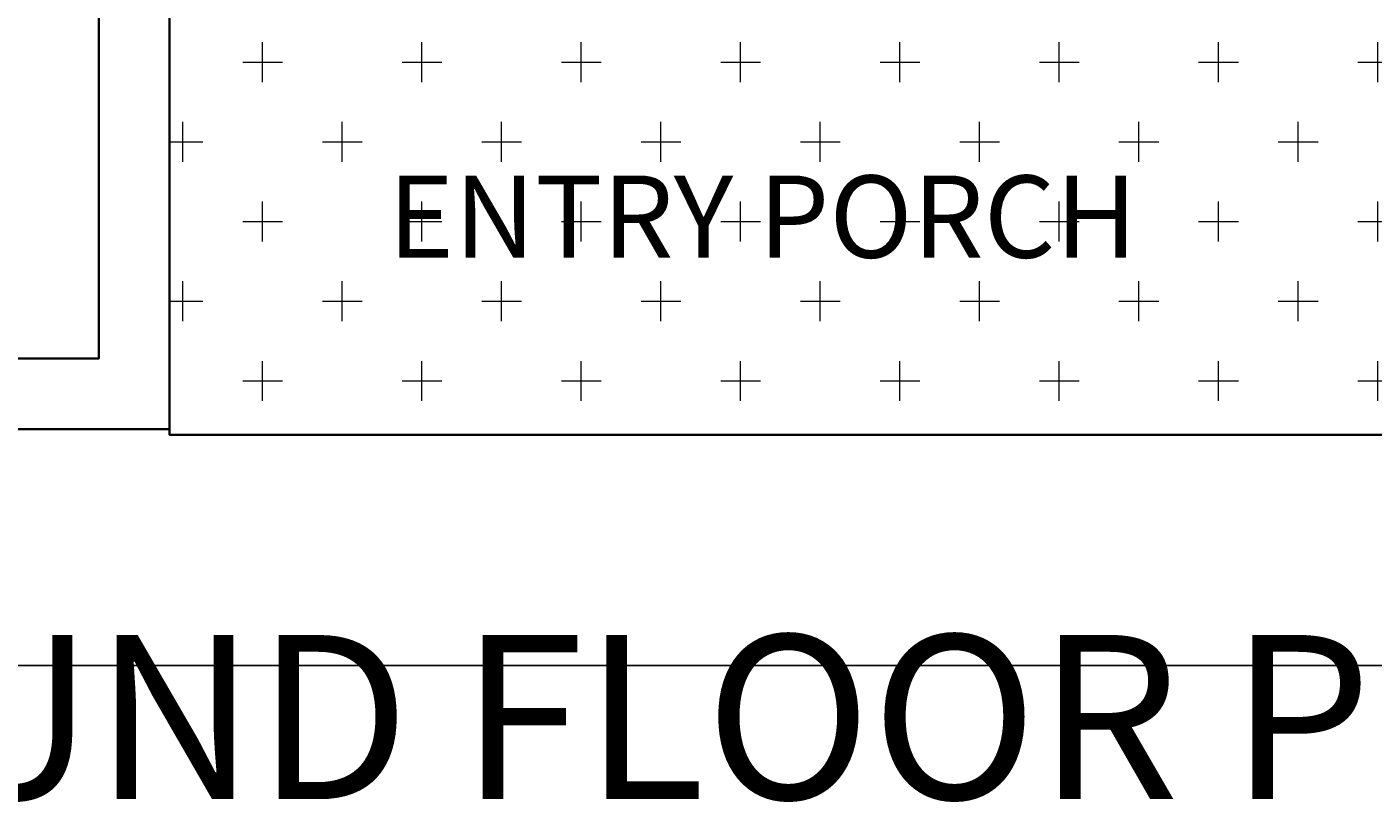
# Model space of a CAD drawing. Units: millimetres. Extents: x 19292 to 100733, y 12374 to 26974.
# Tile 2 of 24: x 26744 to 31036, y 12374 to 14845. Entities that reach past the tile are written whole.
import ezdxf

# ---------------------------------------------------------------- set-up
doc = ezdxf.new("R2010")
doc.units = ezdxf.units.MM
for name, color, linetype, lineweight in [('A-ANNO-DIMS', 2, 'Continuous', 18), ('A-ANNO-TEXT', 7, 'Continuous', 35), ('A-AREA-IDEN', 3, 'Continuous', 25), ('A-FLOR-PATT', 252, 'Continuous', 13), ('A-WALL', 7, 'Continuous', 35)]:
    doc.layers.add(name, color=color, linetype=linetype, lineweight=lineweight)
doc.styles.get("Standard").update_dxf_attribs({"font": 'arial.ttf'})
doc.dimstyles.get("Standard").update_dxf_attribs({"dimtxt": 0.18, "dimasz": 0.18, "dimexe": 0.18, "dimexo": 0.0625, "dimgap": 0.09, "dimtad": 0, "dimtih": 1, "dimtoh": 1, "dimdec": 4, "dimzin": 0, "dimdsep": 46, "dimtxsty": 'Standard', "dimcen": 0.09, "dimadec": 0, "dimazin": 0, "dimtfac": 1, "dimtdec": 4, "dimtofl": 0, "dimtmove": 0, "dimatfit": 3, "dimfxl": 1, "dimtolj": 1, "dimtzin": 0, "dimarcsym": 0})

# ---------------------------------------------------------------- blocks, each defined once
blk = doc.blocks.new('*D71')
at = {"layer": 'A-ANNO-DIMS', "color": 0, "lineweight": -2, "transparency": 16777216}
for p, q in [((26973.8, 17387.7), (26278.6, 17387.7)), ((26278.8, 17387.6), (26278.8, 15587.9)), ((26278.8, 13787.9), (26278.8, 15587.6)), ((26973.8, 13787.7), (26278.6, 13787.7))]:
    blk.add_line(p, q, dxfattribs=at)
at = {"layer": 'A-ANNO-DIMS', "color": 0, "transparency": 16777216}
for points in [[(26278.8, 17387.6), (26278.8, 17387.6), (26278.8, 17387.7)], [(26278.8, 13787.9), (26278.8, 13787.9), (26278.8, 13787.7)]]:
    blk.add_solid(points, dxfattribs=at)
at = {"layer": 'Defpoints', "color": 0, "transparency": 16777216}
for p in [(26278.8, 17387.7), (26973.8, 17387.7), (26973.8, 13787.7)]:
    blk.add_point(p, dxfattribs=at)
at = {"layer": 'A-ANNO-DIMS', "color": 0, "transparency": 16777216, "insert": (26278.8, 15587.7), "char_height": 0.18, "attachment_point": 5}
blk.add_mtext('\\A1;3600', dxfattribs=at)
blk = doc.blocks.new('*D79')
at = {"layer": 'A-ANNO-DIMS', "color": 0, "lineweight": -2, "transparency": 16777216}
for p, q in [((22694.1, 22860.7), (22694.1, 12808.8)), ((36144.2, 15985.7), (36144.2, 12808.8)), ((22694.3, 12809), (29418.7, 12809)), ((36144, 12809), (29419.6, 12809))]:
    blk.add_line(p, q, dxfattribs=at)
at = {"layer": 'A-ANNO-DIMS', "color": 0, "transparency": 16777216}
for points in [[(22694.3, 12809), (22694.3, 12809), (22694.1, 12809)], [(36144, 12809), (36144, 12809), (36144.2, 12809)]]:
    blk.add_solid(points, dxfattribs=at)
at = {"layer": 'Defpoints', "color": 0, "transparency": 16777216}
for p in [(22694.1, 22860.7), (36144.2, 15985.7), (36144.2, 12809)]:
    blk.add_point(p, dxfattribs=at)
at = {"layer": 'A-ANNO-DIMS', "color": 0, "transparency": 16777216, "insert": (29419.2, 12809), "char_height": 0.18, "attachment_point": 5}
blk.add_mtext('\\A1;13450', dxfattribs=at)
blk = doc.blocks.new('*D82')
at = {"layer": 'A-ANNO-DIMS', "color": 0, "lineweight": -2, "transparency": 16777216}
for p, q in [((27198.8, 13562.8), (27198.8, 23555.9)), ((27199, 23555.7), (29296.4, 23555.7)), ((31394.6, 23555.7), (29297.2, 23555.7)), ((31394.8, 13544.1), (31394.8, 23555.9))]:
    blk.add_line(p, q, dxfattribs=at)
at = {"layer": 'A-ANNO-DIMS', "color": 0, "transparency": 16777216}
for points in [[(27199, 23555.8), (27199, 23555.7), (27198.8, 23555.7)], [(31394.6, 23555.8), (31394.6, 23555.7), (31394.8, 23555.7)]]:
    blk.add_solid(points, dxfattribs=at)
at = {"layer": 'Defpoints', "color": 0, "transparency": 16777216}
for p in [(31394.8, 23555.7), (27198.8, 13562.7), (31394.8, 13544)]:
    blk.add_point(p, dxfattribs=at)
at = {"layer": 'A-ANNO-DIMS', "color": 0, "transparency": 16777216, "insert": (29296.8, 23555.7), "char_height": 0.18, "attachment_point": 5}
blk.add_mtext('\\A1;4196', dxfattribs=at)

msp = doc.modelspace()

# ---------------------------------------------------------------- hatches: boundary and pattern name
at = {"layer": 'A-FLOR-PATT'}
h = msp.add_hatch(dxfattribs=at)
h.set_pattern_fill('CROSS', color=256, scale=40)
h.paths.add_polyline_path([(31394.799, 14906.403), (31051.542, 14906.403), (29468.571, 14906.403), (27198.815, 14906.403), (27198.815, 13543.993), (31394.799, 13543.993)])
h.paths.add_polyline_path([(27828.096, 14036.581), (30629.164, 14036.581), (30629.164, 14443.478), (27828.096, 14443.478)], flags=24)

# ---------------------------------------------------------------- linework, layer by layer
at = {"layer": 'A-WALL'}
for points in [[(29548.571, 14906.403), (27198.815, 14906.403), (27198.815, 13562.748), (23348.815, 13562.748), (23348.815, 19010.725), (22694.132, 19010.725), (22694.132, 22860.725), (28369.132, 22860.725), (28369.132, 21460.725), (31169.132, 21460.725), (31169.132, 22460.725), (34419.132, 22460.725), (34419.132, 22208.026)], [(25756.145, 17387.748), (23573.815, 17387.748), (23573.815, 13787.748), (26973.815, 13787.748), (26973.815, 17387.748), (26656.145, 17387.748)], [(31051.542, 14906.403), (31394.799, 14906.403), (31394.799, 13543.993), (27198.815, 13543.993), (27198.815, 14906.403), (29548.571, 14906.403)]]:
    msp.add_lwpolyline(points, dxfattribs=at)

# ---------------------------------------------------------------- texts
at = {"layer": 'A-ANNO-TEXT'}
msp.add_text('GROUND FLOOR PLAN', height=523.26848, dxfattribs=at).set_placement((24968.619, 12383.031))
at = {"layer": 'A-AREA-IDEN'}
msp.add_text('ENTRY PORCH', height=262.14473, dxfattribs=at).set_placement((27895.912, 14108.868))

# ---------------------------------------------------------------- dimensions: what is measured, and where the dimension line sits
at = {"layer": 'A-ANNO-DIMS'}
for base, p1, p2, picture, middle in [((31394.799, 23555.725), (27198.815, 13562.748), (31394.799, 13543.993), '*D82', (29296.807, 23555.725)), ((36144.169, 12808.993), (22694.132, 22860.725), (36144.169, 15985.725), '*D79', (29419.151, 12808.993))]:
    dim = msp.add_linear_dim(base=base, p1=p1, p2=p2, dimstyle='Standard', override={"dimdec": 0, "dimlfac": 1, "dimrnd": 0, "dimzin": 0, "dimdsep": 46, "dimlunit": 2}, dxfattribs=at)
    dim.commit()
    dim.dimension.update_dxf_attribs({"geometry": picture, "text_midpoint": middle})
dim = msp.add_linear_dim(base=(26278.815, 17387.748), p1=(26973.815, 13787.748), p2=(26973.815, 17387.748), angle=90, dimstyle='Standard', override={"dimdec": 0, "dimlfac": 1, "dimrnd": 0, "dimzin": 0, "dimdsep": 46, "dimlunit": 2}, dxfattribs=at)
dim.commit()
dim.dimension.update_dxf_attribs({"geometry": '*D71', "text_midpoint": (26278.815, 15587.748)})

doc.saveas('drawing.dxf')
